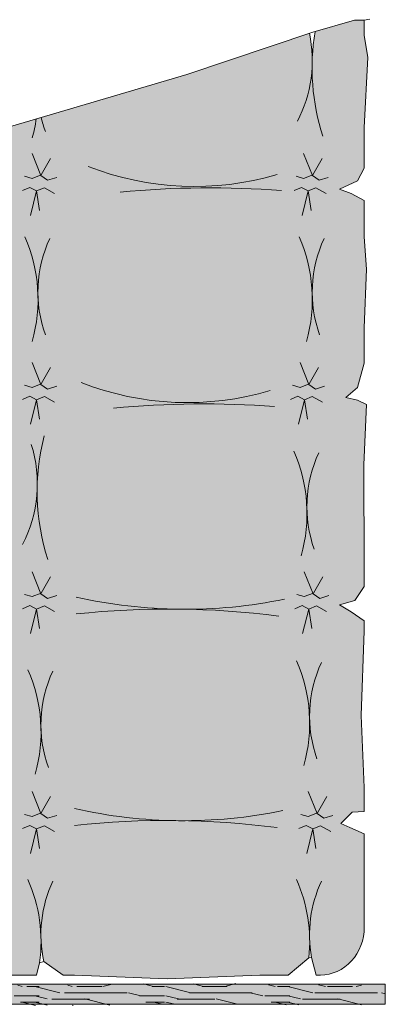
# Model space of a CAD drawing. Units: inches. Extents: x 1994 to 3075, y 3517 to 3950.
# Tile 45 of 58: x 1994.66748 to 1994.68355, y 3553.69193 to 3553.73529. Entities that reach past the tile are written whole.
import ezdxf

# ---------------------------------------------------------------- set-up
doc = ezdxf.new("R2010")
doc.units = ezdxf.units.IN
doc.layers.add('A-FURN-REFR', color=8, linetype='Continuous', lineweight=13)
doc.layers.add('A-FURN-REFR-PATT', color=8, linetype='Continuous', lineweight=13)

msp = doc.modelspace()

# ---------------------------------------------------------------- hatches: boundary and pattern name
at = {"layer": 'A-FURN-REFR-PATT'}
h = msp.add_hatch(color=256, dxfattribs=at)
h.set_gradient(color1=(238, 215, 180), color2=(243, 226, 201), one_color=1, tint=0.87)
edge = h.paths.add_edge_path()
edge.add_line((1994.681542, 3553.709525), (1994.682048, 3553.709217))
edge.add_line((1994.682048, 3553.709217), (1994.682631, 3553.708815))
edge.add_line((1994.682631, 3553.708815), (1994.682631, 3553.708383))
edge.add_line((1994.682631, 3553.708383), (1994.682498, 3553.704652))
edge.add_line((1994.682498, 3553.704652), (1994.682631, 3553.701474))
edge.add_line((1994.682631, 3553.701474), (1994.682631, 3553.700426))
edge.add_line((1994.682631, 3553.700426), (1994.682104, 3553.700396))
edge.add_line((1994.682104, 3553.700396), (1994.681598, 3553.699902))
edge.add_line((1994.681598, 3553.699902), (1994.681992, 3553.699717))
edge.add_line((1994.681992, 3553.699717), (1994.682631, 3553.699439))
edge.add_line((1994.682631, 3553.699439), (1994.682631, 3553.695334))
edge.add_ellipse((1994.680709, 3553.695334), major_axis=(0, 0.002111), ratio=0.910403, start_angle=180, end_angle=270, ccw=False)
edge.add_line((1994.680709, 3553.693223), (1994.680522, 3553.693223))
edge.add_line((1994.680522, 3553.693223), (1994.680314, 3553.694))
edge.add_ellipse((1994.68491, 3553.694998), major_axis=(0, 0.005146), ratio=0.910403, start_angle=92.3431, end_angle=102.2543, ccw=False)
edge.add_ellipse((1994.674568, 3553.694683), major_axis=(0, 0.006219), ratio=0.910403, start_angle=-88.7485, end_angle=-87.76)
edge.add_ellipse((1994.68491, 3553.694998), major_axis=(0, 0.005146), ratio=0.910403, start_angle=91.1484, end_angle=92.3431)
edge.add_ellipse((1994.674568, 3553.694683), major_axis=(0, 0.006219), ratio=0.910403, start_angle=262.8125, end_angle=271.2515, ccw=False)
edge.add_line((1994.680193, 3553.693973), (1994.679278, 3553.693223))
edge.add_line((1994.679278, 3553.693223), (1994.678042, 3553.693223))
edge.add_line((1994.678042, 3553.693223), (1994.673955, 3553.693055))
edge.add_line((1994.673955, 3553.693055), (1994.669892, 3553.693223))
edge.add_line((1994.669892, 3553.693223), (1994.669387, 3553.693223))
edge.add_line((1994.669387, 3553.693223), (1994.668536, 3553.693813))
edge.add_ellipse((1994.673095, 3553.694999), major_axis=(0, 0.005146), ratio=0.910403, start_angle=92.3431, end_angle=104.5922, ccw=False)
edge.add_ellipse((1994.662753, 3553.694684), major_axis=(0, 0.006219), ratio=0.910403, start_angle=-88.7485, end_angle=-87.76)
edge.add_ellipse((1994.673095, 3553.694999), major_axis=(0, 0.005146), ratio=0.910403, start_angle=91.1484, end_angle=92.3431)
edge.add_ellipse((1994.662753, 3553.694684), major_axis=(0, 0.006219), ratio=0.910403, start_angle=260.6759, end_angle=271.2515, ccw=False)
edge.add_line((1994.668352, 3553.693765), (1994.66822, 3553.693223))
edge.add_line((1994.66822, 3553.693223), (1994.666295, 3553.693223))
edge.add_line((1994.666295, 3553.693223), (1994.664702, 3553.693298))
edge.add_line((1994.664702, 3553.693298), (1994.660712, 3553.693051))
edge.add_line((1994.660712, 3553.693051), (1994.65764, 3553.693223))
edge.add_line((1994.65764, 3553.693223), (1994.656797, 3553.693223))
edge.add_line((1994.656797, 3553.693223), (1994.656116, 3553.693819))
edge.add_ellipse((1994.660616, 3553.695249), major_axis=(0, 0.005146), ratio=0.910403, start_angle=92.3431, end_angle=107.6246, ccw=False)
edge.add_ellipse((1994.650274, 3553.694934), major_axis=(0, 0.006219), ratio=0.910403, start_angle=-88.7485, end_angle=-87.76)
edge.add_ellipse((1994.660616, 3553.695249), major_axis=(0, 0.005146), ratio=0.910403, start_angle=91.1484, end_angle=92.3431)
edge.add_ellipse((1994.650274, 3553.694934), major_axis=(0, 0.006219), ratio=0.910403, start_angle=257.752, end_angle=271.2515, ccw=False)
edge.add_line((1994.655829, 3553.693728), (1994.654998, 3553.693223))
edge.add_line((1994.654998, 3553.693223), (1994.649752, 3553.692989))
edge.add_line((1994.649752, 3553.692989), (1994.644994, 3553.693223))
edge.add_line((1994.644994, 3553.693223), (1994.643952, 3553.693223))
edge.add_ellipse((1994.651853, 3553.695067), major_axis=(0, 0.008872), ratio=0.910403, start_angle=89.8354, end_angle=103.1369, ccw=False)
edge.add_ellipse((1994.638929, 3553.695405), major_axis=(0, 0.005332), ratio=0.910403, start_angle=266.2788, end_angle=270.7223)
edge.add_ellipse((1994.651853, 3553.695067), major_axis=(0, 0.008872), ratio=0.910403, start_angle=87.1651, end_angle=89.8354)
edge.add_ellipse((1994.638929, 3553.695405), major_axis=(0, 0.005332), ratio=0.910403, start_angle=243.7698, end_angle=266.2788, ccw=False)
edge.add_line((1994.643359, 3553.693223), (1994.642545, 3553.693223))
edge.add_line((1994.642545, 3553.693223), (1994.641153, 3553.693113))
edge.add_line((1994.641153, 3553.693113), (1994.636432, 3553.693359))
edge.add_line((1994.636432, 3553.693359), (1994.633777, 3553.693223))
edge.add_line((1994.633777, 3553.693223), (1994.63245, 3553.693223))
edge.add_line((1994.63245, 3553.693223), (1994.632375, 3553.693314))
edge.add_ellipse((1994.640193, 3553.695548), major_axis=(0, 0.008872), ratio=0.910403, start_angle=89.8354, end_angle=105.9456, ccw=False)
edge.add_ellipse((1994.627269, 3553.695886), major_axis=(0, 0.005332), ratio=0.910403, start_angle=266.2788, end_angle=270.7223)
edge.add_ellipse((1994.640193, 3553.695548), major_axis=(0, 0.008872), ratio=0.910403, start_angle=87.1651, end_angle=89.8354)
edge.add_ellipse((1994.627269, 3553.695886), major_axis=(0, 0.005332), ratio=0.910403, start_angle=237.8324, end_angle=266.2788, ccw=False)
edge.add_ellipse((1994.6317, 3553.695334), major_axis=(0, 0.002111), ratio=0.910403, start_angle=90, end_angle=174.0631, ccw=False)
edge.add_line((1994.629778, 3553.695334), (1994.629737, 3553.696763))
edge.add_line((1994.629737, 3553.696763), (1994.629778, 3553.698454))
edge.add_line((1994.629778, 3553.698454), (1994.629778, 3553.699441))
edge.add_line((1994.629778, 3553.699441), (1994.629962, 3553.700094))
edge.add_line((1994.629962, 3553.700094), (1994.630637, 3553.700403))
edge.add_line((1994.630637, 3553.700403), (1994.630075, 3553.700834))
edge.add_line((1994.630075, 3553.700834), (1994.629778, 3553.701292))
edge.add_line((1994.629778, 3553.701292), (1994.629778, 3553.702155))
edge.add_line((1994.629778, 3553.702155), (1994.630018, 3553.703363))
edge.add_line((1994.630018, 3553.703363), (1994.630018, 3553.706016))
edge.add_line((1994.630018, 3553.706016), (1994.629778, 3553.708015))
edge.add_line((1994.629778, 3553.708015), (1994.629778, 3553.70894))
edge.add_line((1994.629778, 3553.70894), (1994.630187, 3553.709347))
edge.add_line((1994.630187, 3553.709347), (1994.630918, 3553.70947))
edge.add_line((1994.630918, 3553.70947), (1994.630299, 3553.709902))
edge.add_line((1994.630299, 3553.709902), (1994.629778, 3553.710112))
edge.add_line((1994.629778, 3553.710112), (1994.629778, 3553.712086))
edge.add_line((1994.629778, 3553.712086), (1994.629962, 3553.713788))
edge.add_line((1994.629962, 3553.713788), (1994.629778, 3553.716158))
edge.add_line((1994.629778, 3553.716158), (1994.629778, 3553.718502))
edge.add_line((1994.629778, 3553.718502), (1994.630187, 3553.718908))
edge.add_line((1994.630187, 3553.718908), (1994.629778, 3553.719365))
edge.add_line((1994.629778, 3553.719365), (1994.629778, 3553.72115))
edge.add_line((1994.629778, 3553.72115), (1994.630322, 3553.72115))
edge.add_line((1994.630322, 3553.72115), (1994.634865, 3553.721849))
edge.add_line((1994.634865, 3553.721849), (1994.639494, 3553.724204))
edge.add_line((1994.639494, 3553.724204), (1994.643653, 3553.725608))
edge.add_ellipse((1994.63891, 3553.72447), major_axis=(0, 0.005332), ratio=0.910403, start_angle=270.7223, end_angle=283.4893, ccw=False)
edge.add_ellipse((1994.651833, 3553.724132), major_axis=(0, 0.008872), ratio=0.910403, start_angle=87.1651, end_angle=89.8354)
edge.add_ellipse((1994.63891, 3553.72447), major_axis=(0, 0.005332), ratio=0.910403, start_angle=266.2788, end_angle=270.7223)
edge.add_ellipse((1994.651833, 3553.724132), major_axis=(0, 0.008872), ratio=0.910403, start_angle=438.9501, end_angle=447.1651, ccw=False)
edge.add_line((1994.643881, 3553.725685), (1994.643897, 3553.72569))
edge.add_line((1994.643897, 3553.72569), (1994.649542, 3553.726806))
edge.add_line((1994.649542, 3553.726806), (1994.655977, 3553.727797))
edge.add_line((1994.655977, 3553.727797), (1994.658348, 3553.728382))
edge.add_ellipse((1994.662052, 3553.754177), major_axis=(0, 0.026115), ratio=0.910403, start_angle=171.8281, end_angle=180.2609)
edge.add_ellipse((1994.661314, 3553.682223), major_axis=(0, 0.04585), ratio=0.910403, start_angle=-1.0711, end_angle=-0.1044)
edge.add_ellipse((1994.662052, 3553.754177), major_axis=(0, 0.026115), ratio=0.910403, start_angle=171.8281, end_angle=178.5636, ccw=False)
edge.add_line((1994.658348, 3553.728382), (1994.666025, 3553.730275))
edge.add_line((1994.666025, 3553.730275), (1994.67483, 3553.732877))
edge.add_line((1994.67483, 3553.732877), (1994.680219, 3553.734687))
edge.add_ellipse((1994.675489, 3553.733489), major_axis=(0, 0.005332), ratio=0.910403, start_angle=270.7223, end_angle=284.2178, ccw=False)
edge.add_ellipse((1994.688412, 3553.73315), major_axis=(0, 0.008872), ratio=0.910403, start_angle=87.1651, end_angle=89.8354)
edge.add_ellipse((1994.675489, 3553.733489), major_axis=(0, 0.005332), ratio=0.910403, start_angle=266.2788, end_angle=270.7223)
edge.add_ellipse((1994.688412, 3553.73315), major_axis=(0, 0.008872), ratio=0.910403, start_angle=438.5005, end_angle=447.1651, ccw=False)
edge.add_line((1994.68047, 3553.734766), (1994.682205, 3553.735263))
edge.add_line((1994.682205, 3553.735263), (1994.682631, 3553.735263))
edge.add_line((1994.682631, 3553.735263), (1994.682631, 3553.734609))
edge.add_line((1994.682631, 3553.734609), (1994.682783, 3553.733623))
edge.add_line((1994.682783, 3553.733623), (1994.682631, 3553.730537))
edge.add_line((1994.682631, 3553.730537), (1994.682631, 3553.728749))
edge.add_line((1994.682631, 3553.728749), (1994.682334, 3553.728195))
edge.add_line((1994.682334, 3553.728195), (1994.681547, 3553.727824))
edge.add_line((1994.681547, 3553.727824), (1994.682053, 3553.727639))
edge.add_line((1994.682053, 3553.727639), (1994.682631, 3553.72733))
edge.add_line((1994.682631, 3553.72733), (1994.682631, 3553.725726))
edge.add_line((1994.682631, 3553.725726), (1994.682727, 3553.724308))
edge.add_line((1994.682727, 3553.724308), (1994.682631, 3553.721716))
edge.add_line((1994.682631, 3553.721716), (1994.682631, 3553.720165))
edge.add_line((1994.682631, 3553.720165), (1994.682329, 3553.719086))
edge.add_line((1994.682329, 3553.719086), (1994.681823, 3553.718654))
edge.add_line((1994.681823, 3553.718654), (1994.682329, 3553.718531))
edge.add_line((1994.682329, 3553.718531), (1994.682722, 3553.718346))
edge.add_line((1994.682722, 3553.718346), (1994.68261, 3553.715693))
edge.add_line((1994.68261, 3553.715693), (1994.682631, 3553.711159))
edge.add_line((1994.682631, 3553.711159), (1994.682631, 3553.710327))
edge.add_line((1994.682631, 3553.710327), (1994.682217, 3553.70971))
edge.add_line((1994.682217, 3553.70971), (1994.681542, 3553.709525))
edge = h.paths.add_edge_path(flags=16)
edge.add_ellipse((1994.674017, 3553.663488), major_axis=(0, 0.04585), ratio=0.910403, start_angle=-1.0711, end_angle=-0.1044)
edge.add_ellipse((1994.674755, 3553.735442), major_axis=(0, 0.026115), ratio=0.910403, start_angle=178.5636, end_angle=180.2609)
h.paths.add_polyline_path([(1994.668419, 3553.710039), (1994.668385, 3553.710026), (1994.668404, 3553.710013)], flags=16)
edge = h.paths.add_edge_path(flags=16)
edge.add_ellipse((1994.663397, 3553.714852), major_axis=(0, 0.005332), ratio=0.910403, start_angle=266.2788, end_angle=270.7223)
edge.add_ellipse((1994.67632, 3553.714514), major_axis=(0, 0.008872), ratio=0.910403, start_angle=87.1651, end_angle=89.8354)
edge = h.paths.add_edge_path(flags=16)
edge.add_ellipse((1994.662753, 3553.703926), major_axis=(0, 0.006219), ratio=0.910403, start_angle=-88.7485, end_angle=-87.76)
edge.add_ellipse((1994.673095, 3553.704241), major_axis=(0, 0.005146), ratio=0.910403, start_angle=91.1484, end_angle=92.3431)
h.paths.add_polyline_path([(1994.680357, 3553.710026), (1994.680376, 3553.710013), (1994.680391, 3553.710039)], flags=16)
edge = h.paths.add_edge_path(flags=16)
edge.add_ellipse((1994.684791, 3553.713857), major_axis=(0, 0.005146), ratio=0.910403, start_angle=91.1484, end_angle=92.3431)
edge.add_ellipse((1994.67445, 3553.713542), major_axis=(0, 0.006219), ratio=0.910403, start_angle=-88.7485, end_angle=-87.76)
h.paths.add_polyline_path([(1994.668404, 3553.719229), (1994.668419, 3553.719256), (1994.668385, 3553.719242)], flags=16)
edge = h.paths.add_edge_path(flags=16)
edge.add_ellipse((1994.68491, 3553.704625), major_axis=(0, 0.005146), ratio=0.910403, start_angle=91.1484, end_angle=92.3431)
edge.add_ellipse((1994.674568, 3553.70431), major_axis=(0, 0.006219), ratio=0.910403, start_angle=-88.7485, end_angle=-87.76)
edge = h.paths.add_edge_path(flags=16)
edge.add_ellipse((1994.662353, 3553.744655), major_axis=(0, 0.026115), ratio=0.910403, start_angle=178.5636, end_angle=180.2609)
edge.add_ellipse((1994.661615, 3553.6727), major_axis=(0, 0.04585), ratio=0.910403, start_angle=-1.0711, end_angle=-0.1044)
edge = h.paths.add_edge_path(flags=16)
edge.add_ellipse((1994.662621, 3553.722979), major_axis=(0, 0.006219), ratio=0.910403, start_angle=-88.7485, end_angle=-87.76)
edge.add_ellipse((1994.672963, 3553.723294), major_axis=(0, 0.005146), ratio=0.910403, start_angle=91.1484, end_angle=92.3431)
h.paths.add_polyline_path([(1994.68017, 3553.719242), (1994.680189, 3553.719229), (1994.680204, 3553.719256)], flags=16)
h.paths.add_polyline_path([(1994.668419, 3553.70036), (1994.668385, 3553.700347), (1994.668404, 3553.700334)], flags=16)
edge = h.paths.add_edge_path(flags=16)
edge.add_ellipse((1994.673942, 3553.654177), major_axis=(0, 0.04585), ratio=0.910403, start_angle=-1.0711, end_angle=-0.1044)
edge.add_ellipse((1994.67468, 3553.726132), major_axis=(0, 0.026115), ratio=0.910403, start_angle=178.5636, end_angle=180.2609)
edge = h.paths.add_edge_path(flags=16)
edge.add_ellipse((1994.685026, 3553.723294), major_axis=(0, 0.005146), ratio=0.910403, start_angle=91.1484, end_angle=92.3431)
edge.add_ellipse((1994.674684, 3553.722979), major_axis=(0, 0.006219), ratio=0.910403, start_angle=-88.7485, end_angle=-87.76)
h.paths.add_polyline_path([(1994.680569, 3553.70036), (1994.680535, 3553.700347), (1994.680554, 3553.700334)], flags=16)
h.paths.add_polyline_path([(1994.656068, 3553.710085), (1994.656034, 3553.710071), (1994.656052, 3553.710058)], flags=16)
h.paths.add_polyline_path([(1994.668404, 3553.728426), (1994.668419, 3553.728453), (1994.668385, 3553.728439)], flags=16)
edge = h.paths.add_edge_path(flags=16)
edge.add_ellipse((1994.650317, 3553.713896), major_axis=(0, 0.006219), ratio=0.910403, start_angle=-88.7485, end_angle=-87.76)
edge.add_ellipse((1994.660659, 3553.714211), major_axis=(0, 0.005146), ratio=0.910403, start_angle=91.1484, end_angle=92.3431)
edge = h.paths.add_edge_path(flags=16)
edge.add_ellipse((1994.650274, 3553.70431), major_axis=(0, 0.006219), ratio=0.910403, start_angle=-88.7485, end_angle=-87.76)
edge.add_ellipse((1994.660616, 3553.704625), major_axis=(0, 0.005146), ratio=0.910403, start_angle=91.1484, end_angle=92.3431)
h.paths.add_polyline_path([(1994.68033, 3553.728439), (1994.680349, 3553.728426), (1994.680364, 3553.728453)], flags=16)
h.paths.add_polyline_path([(1994.656052, 3553.719229), (1994.656068, 3553.719256), (1994.656034, 3553.719242)], flags=16)
edge = h.paths.add_edge_path(flags=16)
edge.add_ellipse((1994.649569, 3553.663672), major_axis=(0, 0.04585), ratio=0.910403, start_angle=-1.0711, end_angle=-0.1044)
edge.add_ellipse((1994.650307, 3553.735627), major_axis=(0, 0.026115), ratio=0.910403, start_angle=178.5636, end_angle=180.2609)
h.paths.add_polyline_path([(1994.656068, 3553.700324), (1994.656034, 3553.70031), (1994.656052, 3553.700297)], flags=16)
edge = h.paths.add_edge_path(flags=16)
edge.add_ellipse((1994.650446, 3553.723545), major_axis=(0, 0.006219), ratio=0.910403, start_angle=-88.7485, end_angle=-87.76)
edge.add_ellipse((1994.660788, 3553.72386), major_axis=(0, 0.005146), ratio=0.910403, start_angle=91.1484, end_angle=92.3431)
edge = h.paths.add_edge_path(flags=16)
edge.add_ellipse((1994.64966, 3553.654177), major_axis=(0, 0.04585), ratio=0.910403, start_angle=-1.0711, end_angle=-0.1044)
edge.add_ellipse((1994.650398, 3553.726132), major_axis=(0, 0.026115), ratio=0.910403, start_angle=178.5636, end_angle=180.2609)
h.paths.add_polyline_path([(1994.643774, 3553.710039), (1994.64374, 3553.710026), (1994.643759, 3553.710013)], flags=16)
edge = h.paths.add_edge_path(flags=16)
edge.add_ellipse((1994.638006, 3553.713542), major_axis=(0, 0.006219), ratio=0.910403, start_angle=-88.7485, end_angle=-87.76)
edge.add_ellipse((1994.648347, 3553.713857), major_axis=(0, 0.005146), ratio=0.910403, start_angle=91.1484, end_angle=92.3431)
edge = h.paths.add_edge_path(flags=16)
edge.add_ellipse((1994.638929, 3553.705498), major_axis=(0, 0.005332), ratio=0.910403, start_angle=266.2788, end_angle=270.7223)
edge.add_ellipse((1994.651853, 3553.705159), major_axis=(0, 0.008872), ratio=0.910403, start_angle=87.1651, end_angle=89.8354)
h.paths.add_polyline_path([(1994.643759, 3553.719229), (1994.643774, 3553.719256), (1994.64374, 3553.719242)], flags=16)
h.paths.add_polyline_path([(1994.643774, 3553.700752), (1994.64374, 3553.700739), (1994.643759, 3553.700726)], flags=16)
edge = h.paths.add_edge_path(flags=16)
edge.add_ellipse((1994.637078, 3553.672998), major_axis=(0, 0.04585), ratio=0.910403, start_angle=-1.0711, end_angle=-0.1044)
edge.add_ellipse((1994.637816, 3553.744953), major_axis=(0, 0.026115), ratio=0.910403, start_angle=178.5636, end_angle=180.2609)
edge = h.paths.add_edge_path(flags=16)
edge.add_ellipse((1994.637265, 3553.654177), major_axis=(0, 0.04585), ratio=0.910403, start_angle=-1.0711, end_angle=-0.1044)
edge.add_ellipse((1994.638003, 3553.726132), major_axis=(0, 0.026115), ratio=0.910403, start_angle=178.5636, end_angle=180.2609)
h.paths.add_polyline_path([(1994.632201, 3553.710039), (1994.632167, 3553.710026), (1994.632186, 3553.710013)], flags=16)
edge = h.paths.add_edge_path(flags=16)
edge.add_ellipse((1994.626452, 3553.713542), major_axis=(0, 0.006219), ratio=0.910403, start_angle=-88.7485, end_angle=-87.76)
edge.add_ellipse((1994.636794, 3553.713857), major_axis=(0, 0.005146), ratio=0.910403, start_angle=91.1484, end_angle=92.3431)
edge = h.paths.add_edge_path(flags=16)
edge.add_ellipse((1994.627269, 3553.705498), major_axis=(0, 0.005332), ratio=0.910403, start_angle=266.2788, end_angle=270.7223)
edge.add_ellipse((1994.640193, 3553.705159), major_axis=(0, 0.008872), ratio=0.910403, start_angle=87.1651, end_angle=89.8354)
h.paths.add_polyline_path([(1994.631818, 3553.719229), (1994.631834, 3553.719256), (1994.631799, 3553.719242)], flags=16)
h.paths.add_polyline_path([(1994.631864, 3553.700752), (1994.63183, 3553.700739), (1994.631849, 3553.700726)], flags=16)
msp.add_hatch(color=256, dxfattribs=at).paths.add_polyline_path([(1994.683555, 3553.692818), (1994.629017, 3553.692818), (1994.629017, 3553.691934), (1994.683555, 3553.691934)])
h = msp.add_hatch(dxfattribs=at)
h.set_pattern_fill('LEGNO1', color=256, scale=0.005512, style=0, pattern_type=2)
h.set_pattern_definition([(0, (2000.7131367, 3549.9540566), (0, 0.005511811), [0.0011023622, -0.0016535433, 0.000551181, -0.0022047244]), (0, (2000.716995, 3549.9541944), (0, 0.005511811), [0.001102362, -0.004409449]), (0, (2000.716444, 3549.95447), (0, 0.005511811), [0.000551181, -0.00496063]), (0, (2000.713412, 3549.954608), (0, 0.005511811), [0.0002755906, -0.0038582677, 0.0002755906, -0.0011023622]), (0, (2000.7153414, 3549.9548834), (0, 0.005511811), [0.0011023622, -0.0016535433, 0.0002755906, -0.002480315]), (0, (2000.7139634, 3549.955021), (0, 0.005511811), [0.0008267717, -0.0046850394]), (0, (2000.7153414, 3549.955159), (0, 0.005511811), [0.0016535433, -0.0038582677]), (0, (2000.713688, 3549.955297), (0, 0.005511811), [0.001102362, -0.004409449]), (0, (2000.7158926, 3549.9554346), (0, 0.005511811), [0.0027559055, -0.0027559055]), (0, (2000.714239, 3549.95571), (0, 0.005511811), [0.000551181, -0.0016535433, 0.0011023622, -0.0022047244]), (0, (2000.7180973, 3549.955848), (0, 0.005511811), [0.001102362, -0.004409449]), (0, (2000.716995, 3549.955986), (0, 0.005511811), [0.000551181, -0.00496063]), (0, (2000.7158926, 3549.9561236), (0, 0.005511811), [0.000551181, -0.00496063]), (0, (2000.7131367, 3549.9562614), (0, 0.005511811), [0.001102362, -0.004409449]), (0, (2000.7158926, 3549.956399), (0, 0.005511811), [0.001102362, -0.004409449]), (0, (2000.7158926, 3549.956675), (0, 0.005511811), [0.0011023622, -0.0011023622, 0.0011023622, -0.0022047244]), (0, (2000.71479, 3549.9569503), (0, 0.005511811), [0.000551181, -0.0027559055, 0.0011023622, -0.0011023622]), (0, (2000.7158926, 3549.957088), (0, 0.005511811), [0.0016535433, -0.0038582677]), (0, (2000.7158926, 3549.957364), (0, 0.005511811), [0.001102362, -0.004409449]), (0, (2000.713688, 3549.9575015), (0, 0.005511811), [0.0016535433, -0.0022047244, 0.000551181, -0.0011023622]), (0, (2000.713688, 3549.957777), (0, 0.005511811), [0.0027559055, -0.0027559055]), (0, (2000.716995, 3549.957915), (0, 0.005511811), [0.000551181, -0.00496063]), (0, (2000.7153414, 3549.9580527), (0, 0.005511811), [0.001102362, -0.004409449]), (0, (2000.714239, 3549.9581905), (0, 0.005511811), [0.000551181, -0.0022047244, 0.000551181, -0.0022047244]), (0, (2000.713688, 3549.9583283), (0, 0.005511811), [0.000551181, -0.0016535433, 0.0011023622, -0.0022047244]), (0, (2000.71479, 3549.958466), (0, 0.005511811), [0.000551181, -0.0027559055, 0.000551181, -0.0016535433]), (0, (2000.7158926, 3549.958604), (0, 0.005511811), [0.0016535433, -0.0038582677]), (0, (2000.713688, 3549.9588795), (0, 0.005511811), [0.001102362, -0.004409449]), (0, (2000.716444, 3549.959017), (0, 0.005511811), [0.000551181, -0.00496063]), (0, (2000.717546, 3549.959155), (0, 0.005511811), [0.000551181, -0.00496063]), (14.036243, (2000.7169949, 3549.95447), (0.00551181102, -2e-13), [0.0005677165, -0.022158062]), (14.036243, (2000.7175461, 3549.9557102), (0.00551181102, -2e-13), [0.0005677165, -0.022158062]), (14.036243, (2000.7169949, 3549.9590173), (0.00551181102, -2e-13), [0.0005677165, -0.022158062]), (14.036243, (2000.7153414, 3549.9569503), (0.00551181102, -2e-13), [0.0005677165, -0.022158062]), (14.036243, (2000.7164437, 3549.9577771), (0.00551181102, -2e-13), [0.0005677165, -0.022158062]), (14.036243, (2000.7169949, 3549.9573637), (0.00551181102, -2e-13), [0.0005677165, -0.022158062]), (14.036243, (2000.714239, 3549.9583283), (0.00551181102, -2e-13), [0.0005677165, -0.022158062]), (14.036243, (2000.7164437, 3549.9580527), (0.00551181102, -2e-13), [0.0005677165, -0.022158062]), (14.036243, (2000.7175461, 3549.9559858), (0.00551181102, -2e-13), [0.001135433, -0.0215903454]), (14.036243, (2000.7169949, 3549.9563992), (0.00551181102, -2e-13), [0.001135433, -0.0215903454]), (14.036243, (2000.7169949, 3549.9566748), (0.00551181102, -2e-13), [0.001135433, -0.0215903454]), (165.963757, (2000.7153414, 3549.9548834), (-0.00551181102, -2e-13), [0.0005677165, -0.001135433, 0.0005677165, -0.0204549123]), (165.963757, (2000.714239, 3549.9557102), (-0.00551181102, -2e-13), [0.0005677165, -0.022158062]), (165.963757, (2000.714239, 3549.9581905), (-0.00551181102, -2e-13), [0.001135433, -0.0215903454]), (194.036243, (2000.7169949, 3549.9541944), (-0.00551181102, 2e-13), [0.0005677165, -0.022158062]), (345.963757, (2000.7180973, 3549.9541944), (0.00551181102, 2e-13), [0.0005677165, -0.022158062]), (345.963757, (2000.7164437, 3549.9561236), (0.00551181102, 2e-13), [0.0005677165, -0.022158062]), (345.963757, (2000.7175461, 3549.9570881), (0.00551181102, 2e-13), [0.0005677165, -0.022158062]), (345.963757, (2000.7153414, 3549.9575015), (0.00551181102, 2e-13), [0.0005677165, -0.022158062]), (345.963757, (2000.7147902, 3549.9581905), (0.00551181102, 2e-13), [0.0005677165, -0.022158062]), (345.963757, (2000.7153414, 3549.9584661), (0.00551181102, 2e-13), [0.0005677165, -0.022158062]), (345.963757, (2000.7153414, 3549.9575015), (0.00551181102, 2e-13), [0.0005677165, -0.022158062]), (345.963757, (2000.7169949, 3549.9583283), (0.00551181102, 2e-13), [0.002270866, -0.0204549123]), (345.963757, (2000.7136878, 3549.9546078), (0.00551181102, 2e-13), [0.002270866, -0.0204549123]), (345.963757, (2000.714239, 3549.9550212), (0.00551181102, 2e-13), [0.002270866, -0.0204549123]), (345.963757, (2000.7147902, 3549.9552968), (0.00551181102, 2e-13), [0.0005677165, -0.001135433, 0.001135433, -0.0198871958]), (345.963757, (2000.7147902, 3549.9557102), (0.00551181102, 2e-13), [0.001135433, -0.001135433, 0.001135433, -0.0193194793]), (345.963757, (2000.714239, 3549.9562614), (0.00551181102, 2e-13), [0.002270866, -0.0204549123]), (345.963757, (2000.7136878, 3549.9566748), (0.00551181102, 2e-13), [0.002270866, -0.0204549123]), (345.963757, (2000.7136878, 3549.9569503), (0.00551181102, 2e-13), [0.002270866, -0.0204549123]), (345.963757, (2000.7175461, 3549.9586039), (0.00551181102, 2e-13), [0.0005677165, -0.022158062]), (345.963768, (2000.7180973, 3549.959155), (0.00551181102, 1.06e-09), [0.001135433, -0.0215903454]), (345.963768, (2000.7147902, 3549.9588795), (0.00551181102, 1.06e-09), [0.001135433, -0.0215903454]), (345.963758, (2000.714239, 3549.9540566), (0.00551181102, 1e-10), [0.002270866, -0.0204549123]), (345.963758, (2000.7175461, 3549.9579149), (0.00551181102, 1e-10), [0.0017031496, -0.021022629]), (345.963758, (2000.7180973, 3549.9575015), (0.00551181102, 1e-10), [0.0034062992, -0.0193194793])])
h.paths.add_polyline_path([(1994.683555, 3553.692818), (1994.629017, 3553.692818), (1994.629017, 3553.691934), (1994.683555, 3553.691934)])

# ---------------------------------------------------------------- linework, layer by layer
at = {"layer": 'A-FURN-REFR'}
for p, q in [((1994.680362, 3553.734735), (1994.682205, 3553.735263)), ((1994.682205, 3553.735263), (1994.682631, 3553.735263)), ((1994.682631, 3553.735263), (1994.682871, 3553.735311)), ((1994.682631, 3553.735263), (1994.682631, 3553.734609)), ((1994.67483, 3553.732877), (1994.680362, 3553.734735)), ((1994.682783, 3553.733623), (1994.682631, 3553.734609)), ((1994.682631, 3553.730537), (1994.682783, 3553.733623)), ((1994.666025, 3553.730275), (1994.67483, 3553.732877)), ((1994.682631, 3553.730537), (1994.682631, 3553.728749)), ((1994.668404, 3553.728426), (1994.66802, 3553.729392)), ((1994.668419, 3553.728453), (1994.668833, 3553.729172)), ((1994.680349, 3553.728426), (1994.679965, 3553.729392)), ((1994.680364, 3553.728453), (1994.680777, 3553.729172)), ((1994.682334, 3553.728195), (1994.682631, 3553.728749)), ((1994.667692, 3553.72839), (1994.66802, 3553.728296)), ((1994.66802, 3553.728296), (1994.668419, 3553.728453)), ((1994.668704, 3553.728218), (1994.668404, 3553.728426)), ((1994.669103, 3553.728343), (1994.668704, 3553.728218)), ((1994.679637, 3553.72839), (1994.679965, 3553.728296)), ((1994.679965, 3553.728296), (1994.680364, 3553.728453)), ((1994.680649, 3553.728218), (1994.680349, 3553.728426)), ((1994.681048, 3553.728343), (1994.680649, 3553.728218)), ((1994.681547, 3553.727824), (1994.682334, 3553.728195)), ((1994.667606, 3553.727764), (1994.66792, 3553.727905)), ((1994.66792, 3553.727905), (1994.668219, 3553.727749)), ((1994.668562, 3553.727889), (1994.668219, 3553.727749)), ((1994.669004, 3553.727639), (1994.668562, 3553.727889)), ((1994.679551, 3553.727764), (1994.679865, 3553.727905)), ((1994.679865, 3553.727905), (1994.680164, 3553.727749)), ((1994.680507, 3553.727889), (1994.680164, 3553.727749)), ((1994.680949, 3553.727639), (1994.680507, 3553.727889)), ((1994.682053, 3553.727639), (1994.681547, 3553.727824)), ((1994.668219, 3553.727749), (1994.667949, 3553.726669)), ((1994.668219, 3553.727749), (1994.668348, 3553.726888)), ((1994.680164, 3553.727749), (1994.679894, 3553.726669)), ((1994.680164, 3553.727749), (1994.680293, 3553.726888)), ((1994.682631, 3553.72733), (1994.682053, 3553.727639)), ((1994.682631, 3553.72733), (1994.682631, 3553.725726)), ((1994.682727, 3553.724308), (1994.682631, 3553.725726)), ((1994.682631, 3553.721716), (1994.682727, 3553.724308)), ((1994.682631, 3553.721716), (1994.682631, 3553.720165)), ((1994.668404, 3553.719229), (1994.66802, 3553.720195)), ((1994.668419, 3553.719256), (1994.668833, 3553.719976)), ((1994.680189, 3553.719229), (1994.679805, 3553.720195)), ((1994.680204, 3553.719256), (1994.680617, 3553.719976)), ((1994.682329, 3553.719086), (1994.682631, 3553.720165)), ((1994.667692, 3553.719193), (1994.66802, 3553.719099)), ((1994.66802, 3553.719099), (1994.668419, 3553.719256)), ((1994.668704, 3553.719021), (1994.668404, 3553.719229)), ((1994.669103, 3553.719146), (1994.668704, 3553.719021)), ((1994.679477, 3553.719193), (1994.679805, 3553.719099)), ((1994.679805, 3553.719099), (1994.680204, 3553.719256)), ((1994.680489, 3553.719021), (1994.680189, 3553.719229)), ((1994.680888, 3553.719146), (1994.680489, 3553.719021)), ((1994.681823, 3553.718654), (1994.682329, 3553.719086)), ((1994.667606, 3553.718567), (1994.66792, 3553.718708)), ((1994.66792, 3553.718708), (1994.668219, 3553.718552)), ((1994.668562, 3553.718693), (1994.668219, 3553.718552)), ((1994.669004, 3553.718442), (1994.668562, 3553.718693)), ((1994.679391, 3553.718567), (1994.679705, 3553.718708)), ((1994.679705, 3553.718708), (1994.680004, 3553.718552)), ((1994.680346, 3553.718693), (1994.680004, 3553.718552)), ((1994.680788, 3553.718442), (1994.680346, 3553.718693)), ((1994.682329, 3553.718531), (1994.681823, 3553.718654)), ((1994.668219, 3553.718552), (1994.667949, 3553.717472)), ((1994.668219, 3553.718552), (1994.668348, 3553.717691)), ((1994.680004, 3553.718552), (1994.679733, 3553.717472)), ((1994.680004, 3553.718552), (1994.680133, 3553.717691)), ((1994.682722, 3553.718346), (1994.682329, 3553.718531)), ((1994.68261, 3553.715693), (1994.682722, 3553.718346)), ((1994.682631, 3553.711159), (1994.68261, 3553.715693)), ((1994.668404, 3553.710013), (1994.66802, 3553.710978)), ((1994.680376, 3553.710013), (1994.679992, 3553.710978)), ((1994.682631, 3553.711159), (1994.682631, 3553.710327)), ((1994.668419, 3553.710039), (1994.668833, 3553.710759)), ((1994.680391, 3553.710039), (1994.680804, 3553.710759)), ((1994.66802, 3553.709883), (1994.668419, 3553.710039)), ((1994.668704, 3553.709804), (1994.668404, 3553.710013)), ((1994.679992, 3553.709883), (1994.680391, 3553.710039)), ((1994.680676, 3553.709804), (1994.680376, 3553.710013)), ((1994.682217, 3553.70971), (1994.682631, 3553.710327)), ((1994.667692, 3553.709977), (1994.66802, 3553.709883)), ((1994.669103, 3553.70993), (1994.668704, 3553.709804)), ((1994.679664, 3553.709977), (1994.679992, 3553.709883)), ((1994.681075, 3553.70993), (1994.680676, 3553.709804)), ((1994.681542, 3553.709525), (1994.682217, 3553.70971)), ((1994.667606, 3553.709351), (1994.66792, 3553.709492)), ((1994.66792, 3553.709492), (1994.668219, 3553.709335)), ((1994.668219, 3553.709335), (1994.667949, 3553.708255)), ((1994.668562, 3553.709476), (1994.668219, 3553.709335)), ((1994.668219, 3553.709335), (1994.668348, 3553.708474)), ((1994.669004, 3553.709226), (1994.668562, 3553.709476)), ((1994.679578, 3553.709351), (1994.679892, 3553.709492)), ((1994.679892, 3553.709492), (1994.680191, 3553.709335)), ((1994.680191, 3553.709335), (1994.67992, 3553.708255)), ((1994.680533, 3553.709476), (1994.680191, 3553.709335)), ((1994.680191, 3553.709335), (1994.68032, 3553.708474)), ((1994.680975, 3553.709226), (1994.680533, 3553.709476)), ((1994.682048, 3553.709217), (1994.681542, 3553.709525)), ((1994.682631, 3553.708815), (1994.682048, 3553.709217)), ((1994.682631, 3553.708815), (1994.682631, 3553.708383)), ((1994.682498, 3553.704652), (1994.682631, 3553.708383)), ((1994.682631, 3553.701474), (1994.682498, 3553.704652)), ((1994.682631, 3553.701474), (1994.682631, 3553.700426)), ((1994.668404, 3553.700334), (1994.66802, 3553.701299)), ((1994.668419, 3553.70036), (1994.668833, 3553.70108)), ((1994.680554, 3553.700334), (1994.68017, 3553.701299)), ((1994.680569, 3553.70036), (1994.680983, 3553.70108)), ((1994.667692, 3553.700298), (1994.66802, 3553.700204)), ((1994.66802, 3553.700204), (1994.668419, 3553.70036)), ((1994.668704, 3553.700125), (1994.668404, 3553.700334)), ((1994.669103, 3553.700251), (1994.668704, 3553.700125)), ((1994.679842, 3553.700298), (1994.68017, 3553.700204)), ((1994.68017, 3553.700204), (1994.680569, 3553.70036)), ((1994.680855, 3553.700125), (1994.680554, 3553.700334)), ((1994.681254, 3553.700251), (1994.680855, 3553.700125)), ((1994.681598, 3553.699902), (1994.682104, 3553.700396)), ((1994.682104, 3553.700396), (1994.682631, 3553.700426)), ((1994.667606, 3553.699672), (1994.66792, 3553.699813)), ((1994.66792, 3553.699813), (1994.668219, 3553.699656)), ((1994.668219, 3553.699656), (1994.667949, 3553.698576)), ((1994.668562, 3553.699797), (1994.668219, 3553.699656)), ((1994.668219, 3553.699656), (1994.668348, 3553.698795)), ((1994.669004, 3553.699547), (1994.668562, 3553.699797)), ((1994.679757, 3553.699672), (1994.68007, 3553.699813)), ((1994.68007, 3553.699813), (1994.68037, 3553.699656)), ((1994.68037, 3553.699656), (1994.680099, 3553.698576)), ((1994.680712, 3553.699797), (1994.68037, 3553.699656)), ((1994.68037, 3553.699656), (1994.680498, 3553.698795)), ((1994.681154, 3553.699547), (1994.680712, 3553.699797)), ((1994.681992, 3553.699717), (1994.681598, 3553.699902)), ((1994.682631, 3553.699439), (1994.681992, 3553.699717)), ((1994.682631, 3553.699439), (1994.682631, 3553.695334)), ((1994.679278, 3553.693223), (1994.680193, 3553.693973)), ((1994.680193, 3553.693973), (1994.680314, 3553.694)), ((1994.680314, 3553.694), (1994.680522, 3553.693223)), ((1994.66822, 3553.693223), (1994.668352, 3553.693765)), ((1994.668352, 3553.693765), (1994.668536, 3553.693813)), ((1994.668536, 3553.693813), (1994.669387, 3553.693223)), ((1994.66822, 3553.693223), (1994.666295, 3553.693223)), ((1994.669892, 3553.693223), (1994.669387, 3553.693223)), ((1994.669892, 3553.693223), (1994.673955, 3553.693055)), ((1994.673955, 3553.693055), (1994.678042, 3553.693223)), ((1994.679278, 3553.693223), (1994.678042, 3553.693223)), ((1994.680513, 3553.693223), (1994.680709, 3553.693223)), ((1994.683555, 3553.692818), (1994.629017, 3553.692818)), ((1994.683555, 3553.691934), (1994.683555, 3553.692818)), ((1994.629017, 3553.691934), (1994.683555, 3553.691934))]:
    msp.add_line(p, q, dxfattribs=at)
at = {"layer": 'A-FURN-REFR', "extrusion": (0, 0, -1)}
for centre, major_axis, start_param, end_param in [((1994.688412, 3553.73315), (0, 0.008872), 4.368048, 4.895528), ((1994.675489, 3553.733489), (0, 0.005332), 1.344093, 2.094288), ((1994.662621, 3553.731934), (0, 0.006219), 1.734596, 1.873711), ((1994.672963, 3553.732249), (0, 0.005146), 4.336804, 4.463858), ((1994.675152, 3553.743245), (0, 0.015305), 2.877158, 3.483445), ((1994.675853, 3553.678103), (0, 0.049781), -0.087368, 0.069201), ((1994.662621, 3553.722979), (0, 0.006219), 1.114213, 1.873711), ((1994.672963, 3553.723294), (0, 0.005146), 4.336804, 5.187972), ((1994.674684, 3553.722979), (0, 0.006219), 1.114213, 1.873711), ((1994.685026, 3553.723294), (0, 0.005146), 4.336804, 5.187972), ((1994.67485, 3553.733731), (0, 0.015305), 2.877158, 3.483445), ((1994.675551, 3553.66859), (0, 0.049781), -0.087368, 0.069201), ((1994.67632, 3553.714514), (0, 0.008872), 4.368048, 4.991898), ((1994.663397, 3553.714852), (0, 0.005332), 1.239326, 2.094288), ((1994.67445, 3553.713542), (0, 0.006219), 1.114213, 1.873711), ((1994.684791, 3553.713857), (0, 0.005146), 4.336804, 5.187972), ((1994.674755, 3553.735442), (0, 0.026115), 2.956807, 3.344881), ((1994.674017, 3553.663488), (0, 0.04585), -0.097463, 0.116495), ((1994.674568, 3553.70431), (0, 0.006219), 1.114213, 1.873711), ((1994.68491, 3553.704625), (0, 0.005146), 4.336804, 5.187972), ((1994.662753, 3553.703926), (0, 0.006219), 1.114213, 1.873711), ((1994.673095, 3553.704241), (0, 0.005146), 4.336804, 5.187972), ((1994.67468, 3553.726132), (0, 0.026115), 2.956807, 3.344881), ((1994.673942, 3553.654177), (0, 0.04585), -0.097463, 0.116495), ((1994.662753, 3553.694684), (0, 0.006219), 1.114213, 1.719175), ((1994.674568, 3553.694683), (0, 0.006219), 1.114213, 1.685105), ((1994.673095, 3553.694999), (0, 0.005146), 4.479674, 5.187972), ((1994.68491, 3553.694998), (0, 0.005146), 4.517168, 5.187972), ((1994.680709, 3553.695334), (0, 0.002111), 1.570796, 3.141593)]:
    msp.add_ellipse(centre, major_axis=major_axis, ratio=0.910403, start_param=start_param, end_param=end_param, dxfattribs=at)

doc.saveas('drawing.dxf')
